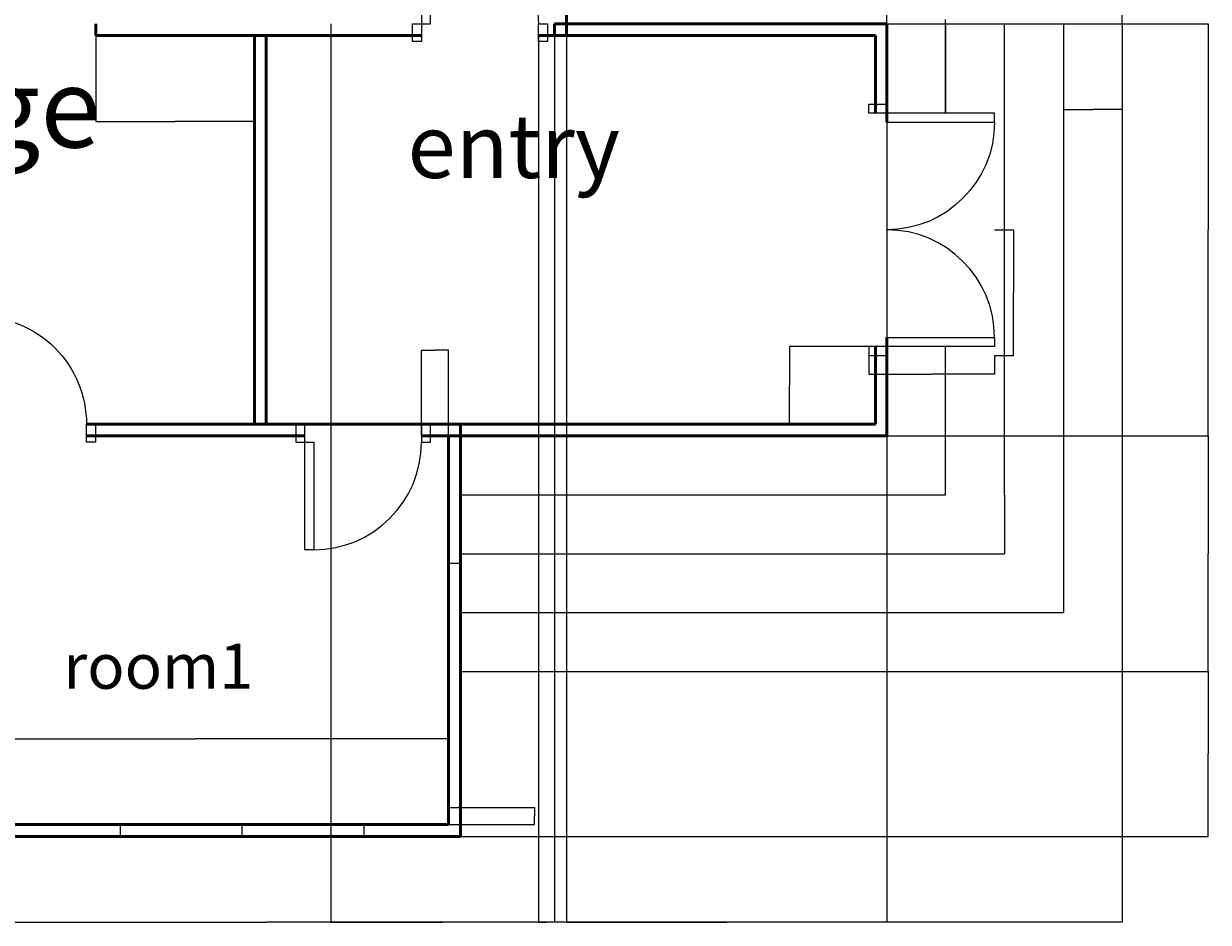
# Model space of a CAD drawing. Units: millimetres. Extents: x 756 to 17937, y 31 to 15590.
# Tile 3 of 6: x 7469 to 17520, y 31 to 7660. Entities that reach past the tile are written whole.
import ezdxf

# ---------------------------------------------------------------- set-up
doc = ezdxf.new("R2010")
doc.units = ezdxf.units.MM
for name, color, linetype, lineweight in [('A-ANNO-DIMS', 2, 'Continuous', 18), ('A-AREA-IDEN', 7, 'Continuous', 25), ('A-DOOR', 3, 'Continuous', 25), ('A-FLOR-STRS', 7, 'Continuous', 25), ('A-GLAZ', 4, 'Continuous', 18), ('A-WALL', 7, 'Continuous', 50)]:
    doc.layers.add(name, color=color, linetype=linetype, lineweight=lineweight)
doc.styles.get("Standard").update_dxf_attribs({"font": 'arial.ttf'})
doc.dimstyles.get("Standard").update_dxf_attribs({"dimtxt": 0.18, "dimasz": 0.18, "dimexe": 0.18, "dimexo": 0.0625, "dimgap": 0.09, "dimtad": 0, "dimtih": 1, "dimtoh": 1, "dimdec": 4, "dimzin": 0, "dimdsep": 46, "dimtxsty": 'Standard', "dimcen": 0.09, "dimadec": 0, "dimazin": 0, "dimtfac": 1, "dimtdec": 4, "dimtofl": 0, "dimtmove": 0, "dimatfit": 3, "dimfxl": 1, "dimtolj": 1, "dimtzin": 0, "dimarcsym": 0})

# ---------------------------------------------------------------- blocks, each defined once
blk = doc.blocks.new('DOOR-SINGLE-914')
for p, q in [((76.2004154520555, 1066.800209260013), (0.0004154520547672, 1066.800209260013)), ((0.0004154520547672, 1066.800209260013), (0.0004154520547672, 914.400209260013)), ((76.2004154520555, 914.400209260013), (76.2004154520555, 1066.800209260013)), ((1143.000415452054, 1066.800209260013), (1066.800415452054, 1066.800209260013)), ((1066.800415452054, 1066.800209260013), (1066.800415452054, 914.400209260013)), ((1143.000415452054, 914.400209260013), (1143.000415452054, 1066.800209260013)), ((0.0004154520547672, 914.400209260013), (76.2004154520555, 914.400209260013)), ((76.2004154520555, 914.400209260013), (152.4004154520562, 914.400209260013)), ((76.2004154520555, 0.0002092600134347), (76.2004154520555, 914.400209260013)), ((152.4004154520562, 914.400209260013), (152.4004154520562, 0.0002092600134347)), ((1066.800415452054, 914.400209260013), (1143.000415452054, 914.400209260013)), ((152.4004154520562, 0.0002092600134347), (76.2004154520555, 0.0002092600134347))]:
    blk.add_line(p, q)
blk.add_arc((152.4004154520562, 914.400209260013), 914.3999999999996, 270, 0)
blk = doc.blocks.new('DOOR-PAIR-LEAF-914')
for p, q in [((152.4003917740337, 76.20024496712995), (152.4003917740337, 152.4002449671306)), ((152.4003917740337, 152.4002449671306), (1066.800391774033, 152.4002449671306)), ((1066.800391774033, 152.4002449671306), (1066.800391774033, 76.20024496712995)), ((152.4003917740337, 76.20024496712995), (0.0003917740341421, 76.20024496712995)), ((0.0003917740341421, 76.20024496712995), (0.0003917740341421, 0.0002449671292197)), ((0.0003917740341421, 0.0002449671292197), (152.4003917740337, 0.0002449671292197)), ((1066.800391774033, 76.20024496712995), (152.4003917740337, 76.20024496712995)), ((152.4003917740337, 0.0002449671292197), (152.4003917740337, 76.20024496712995))]:
    blk.add_line(p, q)
blk.add_arc((152.4003917740337, 152.4002449671306), 914.3999999999996, 0, 90)
blk = doc.blocks.new('WIN-2073')
for p, q in [((8.2799133452e-06, 99.99960647437545), (8.2799133452e-06, -0.0003935256245313)), ((2072.903750917166, 99.99960647437545), (8.2799133452e-06, 99.99960647437545)), ((2072.903750917166, -0.0003935256245313), (2072.903750917166, 99.99960647437545)), ((8.2799133452e-06, -0.0003935256245313), (2072.903750917166, -0.0003935256245313))]:
    blk.add_line(p, q)
blk = doc.blocks.new('*D19')
at = {"layer": 'A-ANNO-DIMS', "color": 0, "lineweight": -2, "transparency": 16777216}
for p, q in [((15706.70389177404, 5910.170244967132), (15866.84139177405, 5910.170244967132)), ((15866.66139177405, 5909.990244967132), (15866.66139177405, 5376.952148104922)), ((15866.66139177405, 4843.550244967131), (15866.66139177405, 5376.588341829341)), ((15706.70389177404, 4843.370244967131), (15866.84139177405, 4843.370244967131))]:
    blk.add_line(p, q, dxfattribs=at)
at = {"layer": 'A-ANNO-DIMS', "color": 0, "transparency": 16777216}
for points in [[(15866.63139177405, 5909.990244967132), (15866.69139177405, 5909.990244967132), (15866.66139177405, 5910.170244967132)], [(15866.63139177405, 4843.550244967131), (15866.69139177405, 4843.550244967131), (15866.66139177405, 4843.370244967131)]]:
    blk.add_solid(points, dxfattribs=at)
at = {"layer": 'Defpoints', "color": 0, "transparency": 16777216}
for p in [(15706.64139177404, 5910.170244967132), (15866.66139177405, 5910.170244967132), (15706.64139177404, 4843.370244967131)]:
    blk.add_point(p, dxfattribs=at)
at = {"layer": 'A-ANNO-DIMS', "color": 0, "transparency": 16777216, "insert": (15866.66139177405, 5376.770244967126), "char_height": 0.18, "attachment_point": 5}
blk.add_mtext('\\A1;PAIRED LEAF 1067 TYP.', dxfattribs=at)
blk = doc.blocks.new('*D20')
at = {"layer": 'A-ANNO-DIMS', "color": 0, "lineweight": -2, "transparency": 16777216}
for p, q in [((14639.84139177403, 4843.30774496713), (14639.84139177403, 4683.170244967128)), ((15706.64139177403, 4843.30774496713), (15706.64139177403, 4683.170244967128)), ((14640.02139177403, 4683.350244967129), (15172.58192383406, 4683.350244967129)), ((15706.46139177403, 4683.350244967129), (15173.90085971401, 4683.350244967129))]:
    blk.add_line(p, q, dxfattribs=at)
at = {"layer": 'A-ANNO-DIMS', "color": 0, "transparency": 16777216}
for points in [[(14640.02139177403, 4683.380244967128), (14640.02139177403, 4683.320244967129), (14639.84139177403, 4683.350244967129)], [(15706.46139177403, 4683.380244967128), (15706.46139177403, 4683.320244967129), (15706.64139177403, 4683.350244967129)]]:
    blk.add_solid(points, dxfattribs=at)
at = {"layer": 'Defpoints', "color": 0, "transparency": 16777216}
for p in [(14639.84139177403, 4843.370244967129), (15706.64139177403, 4843.370244967129), (15706.64139177403, 4683.350244967129)]:
    blk.add_point(p, dxfattribs=at)
at = {"layer": 'A-ANNO-DIMS', "color": 0, "transparency": 16777216, "insert": (15173.24139177403, 4683.350244967129), "char_height": 0.18, "attachment_point": 5}
blk.add_mtext('\\A1;1067 TYP.', dxfattribs=at)
blk = doc.blocks.new('*D43')
at = {"layer": 'A-ANNO-DIMS', "color": 0, "lineweight": -2, "transparency": 16777216}
for p, q in [((16790.928101, 2160.118106), (16790.928101, 30.75060600000006)), ((2274.113703, 760.118106), (2274.113703, 30.75060600000006)), ((2274.293703, 30.930606), (9532.10067689768, 30.930606)), ((16790.748101, 30.930606), (9532.94112710232, 30.930606))]:
    blk.add_line(p, q, dxfattribs=at)
at = {"layer": 'A-ANNO-DIMS', "color": 0, "transparency": 16777216}
for points in [[(2274.293703, 30.960606), (2274.293703, 30.900606), (2274.113703, 30.930606)], [(16790.748101, 30.960606), (16790.748101, 30.900606), (16790.928101, 30.930606)]]:
    blk.add_solid(points, dxfattribs=at)
at = {"layer": 'Defpoints', "color": 0, "transparency": 16777216}
for p in [(16790.928101, 2160.180606), (2274.113703, 760.180606), (16790.928101, 30.930606)]:
    blk.add_point(p, dxfattribs=at)
at = {"layer": 'A-ANNO-DIMS', "color": 0, "transparency": 16777216, "insert": (9532.520901999998, 30.930606), "char_height": 0.18, "attachment_point": 5}
blk.add_mtext('\\A1;14517', dxfattribs=at)
blk = doc.blocks.new('*D46')
at = {"layer": 'A-ANNO-DIMS', "color": 0, "lineweight": -2, "transparency": 16777216}
for p, q in [((6774.113703000001, 860.243106), (6774.113703000001, 1589.610606)), ((6774.293703000001, 1589.430606), (8923.751615687586, 1589.430606)), ((11073.933703, 1589.430606), (8924.475790312415, 1589.430606)), ((11074.113703, 860.243106), (11074.113703, 1589.610606))]:
    blk.add_line(p, q, dxfattribs=at)
at = {"layer": 'A-ANNO-DIMS', "color": 0, "transparency": 16777216}
for points in [[(6774.293703000001, 1589.460606), (6774.293703000001, 1589.400606), (6774.113703000001, 1589.430606)], [(11073.933703, 1589.460606), (11073.933703, 1589.400606), (11074.113703, 1589.430606)]]:
    blk.add_solid(points, dxfattribs=at)
at = {"layer": 'Defpoints', "color": 0, "transparency": 16777216}
for p in [(11074.113703, 1589.430606), (6774.113703000001, 860.1806059999999), (11074.113703, 860.1806059999999)]:
    blk.add_point(p, dxfattribs=at)
at = {"layer": 'A-ANNO-DIMS', "color": 0, "transparency": 16777216, "insert": (8924.113703, 1589.430606), "char_height": 0.18, "attachment_point": 5}
blk.add_mtext('\\A1;4300', dxfattribs=at)
blk = doc.blocks.new('*D47')
at = {"layer": 'A-ANNO-DIMS', "color": 0, "lineweight": -2, "transparency": 16777216}
for p, q in [((16790.99060100001, 2160.180606000001), (17520.35810100001, 2160.180606000001)), ((17520.17810100001, 2160.000606000002), (17520.17810100001, 1460.362509137791)), ((17520.17810100001, 760.3606060000012), (17520.17810100001, 1459.998702862211)), ((11174.176203, 760.1806060000002), (17520.35810100001, 760.1806060000011))]:
    blk.add_line(p, q, dxfattribs=at)
at = {"layer": 'A-ANNO-DIMS', "color": 0, "transparency": 16777216}
for points in [[(17520.14810100001, 2160.000606000002), (17520.20810100001, 2160.000606000002), (17520.17810100001, 2160.180606000001)], [(17520.14810100001, 760.3606060000012), (17520.20810100001, 760.3606060000012), (17520.17810100001, 760.1806060000011)]]:
    blk.add_solid(points, dxfattribs=at)
at = {"layer": 'Defpoints', "color": 0, "transparency": 16777216}
for p in [(16790.92810100001, 2160.180606000001), (17520.17810100001, 2160.180606000001), (11174.113703, 760.1806060000002)]:
    blk.add_point(p, dxfattribs=at)
at = {"layer": 'A-ANNO-DIMS', "color": 0, "transparency": 16777216, "insert": (17520.17810100001, 1460.180605999996), "char_height": 0.18, "attachment_point": 5}
blk.add_mtext('\\A1;1400', dxfattribs=at)
blk = doc.blocks.new('*D48')
at = {"layer": 'A-ANNO-DIMS', "color": 0, "lineweight": -2, "transparency": 16777216}
for p, q in [((14792.303892, 4160.180606000001), (17520.35810100001, 4160.180606000001)), ((17520.17810100001, 4160.000606000001), (17520.17810100001, 3160.362509137792)), ((17520.17810100001, 2160.360606000001), (17520.17810100001, 3159.998702862212)), ((16790.99060100001, 2160.180606000001), (17520.35810100001, 2160.180606000001))]:
    blk.add_line(p, q, dxfattribs=at)
at = {"layer": 'A-ANNO-DIMS', "color": 0, "transparency": 16777216}
for points in [[(17520.14810100001, 4160.000606000001), (17520.20810100001, 4160.000606000001), (17520.17810100001, 4160.180606000001)], [(17520.14810100001, 2160.360606000001), (17520.20810100001, 2160.360606000001), (17520.17810100001, 2160.180606000001)]]:
    blk.add_solid(points, dxfattribs=at)
at = {"layer": 'Defpoints', "color": 0, "transparency": 16777216}
for p in [(14792.241392, 4160.180606000001), (17520.17810100001, 4160.180606000001), (16790.92810100001, 2160.180606000001)]:
    blk.add_point(p, dxfattribs=at)
at = {"layer": 'A-ANNO-DIMS', "color": 0, "transparency": 16777216, "insert": (17520.17810100001, 3160.180605999996), "char_height": 0.18, "attachment_point": 5}
blk.add_mtext('\\A1;2000', dxfattribs=at)
blk = doc.blocks.new('*D49')
at = {"layer": 'A-ANNO-DIMS', "color": 0, "lineweight": -2, "transparency": 16777216}
for p, q in [((14792.303892, 7660.159883000004), (17520.35810100001, 7660.159883000004)), ((17520.17810100001, 7659.979883000004), (17520.17810100001, 5910.352209029333)), ((17520.17810100001, 4160.360606000002), (17520.17810100001, 5909.98827997067)), ((14792.303892, 4160.180606000001), (17520.35810100001, 4160.180606000001))]:
    blk.add_line(p, q, dxfattribs=at)
at = {"layer": 'A-ANNO-DIMS', "color": 0, "transparency": 16777216}
for points in [[(17520.14810100001, 7659.979883000004), (17520.20810100001, 7659.979883000004), (17520.17810100001, 7660.159883000004)], [(17520.14810100001, 4160.360606000002), (17520.20810100001, 4160.360606000002), (17520.17810100001, 4160.180606000001)]]:
    blk.add_solid(points, dxfattribs=at)
at = {"layer": 'Defpoints', "color": 0, "transparency": 16777216}
for p in [(14792.241392, 7660.159883000004), (17520.17810100001, 7660.159883000004), (14792.241392, 4160.180606000001)]:
    blk.add_point(p, dxfattribs=at)
at = {"layer": 'A-ANNO-DIMS', "color": 0, "transparency": 16777216, "insert": (17520.17810100001, 5910.170244499997), "char_height": 0.18, "attachment_point": 5}
blk.add_mtext('\\A1;3500', dxfattribs=at)
blk = doc.blocks.new('*D57')
at = {"layer": 'A-ANNO-DIMS', "color": 0, "lineweight": -2, "transparency": 16777216}
for p, q in [((14792.241392, 7660.097383), (14792.241392, 30.75060599999961)), ((12074.113703, 7560.097383), (12074.113703, 30.75060599999961)), ((12074.293703, 30.930606), (13432.81705636766, 30.930606)), ((14792.061392, 30.930606), (13433.53803863233, 30.930606))]:
    blk.add_line(p, q, dxfattribs=at)
at = {"layer": 'A-ANNO-DIMS', "color": 0, "transparency": 16777216}
for points in [[(12074.293703, 30.960606), (12074.293703, 30.900606), (12074.113703, 30.930606)], [(14792.061392, 30.960606), (14792.061392, 30.900606), (14792.241392, 30.930606)]]:
    blk.add_solid(points, dxfattribs=at)
at = {"layer": 'Defpoints', "color": 0, "transparency": 16777216}
for p in [(14792.241392, 7660.159883), (12074.113703, 7560.159883), (14792.241392, 30.930606)]:
    blk.add_point(p, dxfattribs=at)
at = {"layer": 'A-ANNO-DIMS', "color": 0, "transparency": 16777216, "insert": (13433.1775475, 30.930606), "char_height": 0.18, "attachment_point": 5}
blk.add_mtext('\\A1;2718', dxfattribs=at)
blk = doc.blocks.new('*D58')
at = {"layer": 'A-ANNO-DIMS', "color": 0, "lineweight": -2, "transparency": 16777216}
for p, q in [((14792.241392, 7660.222383), (14792.241392, 8389.589883)), ((14792.421392, 8389.409883), (15791.1295896105, 8389.409883)), ((16790.748101, 8389.409883), (15792.03990338949, 8389.409883)), ((16790.928101, 7660.222383), (16790.928101, 8389.589883))]:
    blk.add_line(p, q, dxfattribs=at)
at = {"layer": 'A-ANNO-DIMS', "color": 0, "transparency": 16777216}
for points in [[(14792.421392, 8389.439883000001), (14792.421392, 8389.379883), (14792.241392, 8389.409883)], [(16790.748101, 8389.439883000001), (16790.748101, 8389.379883), (16790.928101, 8389.409883)]]:
    blk.add_solid(points, dxfattribs=at)
at = {"layer": 'Defpoints', "color": 0, "transparency": 16777216}
for p in [(16790.928101, 8389.409883), (14792.241392, 7660.159883), (16790.928101, 7660.159883)]:
    blk.add_point(p, dxfattribs=at)
at = {"layer": 'A-ANNO-DIMS', "color": 0, "transparency": 16777216, "insert": (15791.5847465, 8389.409883), "char_height": 0.18, "attachment_point": 5}
blk.add_mtext('\\A1;1998.7', dxfattribs=at)
blk = doc.blocks.new('*D59')
at = {"layer": 'A-ANNO-DIMS', "color": 0, "lineweight": -2, "transparency": 16777216}
for p, q in [((16290.928101, 7660.097383), (16290.928101, 6930.729882999999)), ((16790.928101, 7660.097383), (16790.928101, 6930.729883000001)), ((16291.108101, 6930.909882999999), (16540.63956075443, 6930.909883000001)), ((16790.748101, 6930.909883000001), (16541.21664124556, 6930.909883000001))]:
    blk.add_line(p, q, dxfattribs=at)
at = {"layer": 'A-ANNO-DIMS', "color": 0, "transparency": 16777216}
for points in [[(16291.108101, 6930.939882999999), (16291.108101, 6930.879883), (16290.928101, 6930.909882999999)], [(16790.748101, 6930.939883), (16790.748101, 6930.879883000002), (16790.928101, 6930.909883000001)]]:
    blk.add_solid(points, dxfattribs=at)
at = {"layer": 'Defpoints', "color": 0, "transparency": 16777216}
for p in [(16290.928101, 7660.159883), (16790.928101, 7660.159883), (16290.928101, 6930.909882999999)]:
    blk.add_point(p, dxfattribs=at)
at = {"layer": 'A-ANNO-DIMS', "color": 0, "transparency": 16777216, "insert": (16540.928101, 6930.909883000001), "char_height": 0.18, "attachment_point": 5}
blk.add_mtext('\\A1;500', dxfattribs=at)
blk = doc.blocks.new('*D60')
at = {"layer": 'A-ANNO-DIMS', "color": 0, "lineweight": -2, "transparency": 16777216}
for p, q in [((8080.230142000001, 7560.118106), (8080.230142000001, 6830.750605999999)), ((9426.842559999997, 7560.118106), (9426.842559999997, 6830.750605999999)), ((8080.410142000001, 6830.930605999999), (8753.081255502046, 6830.930605999999)), ((9426.662559999999, 6830.930605999999), (8753.991446497952, 6830.930605999999))]:
    blk.add_line(p, q, dxfattribs=at)
at = {"layer": 'A-ANNO-DIMS', "color": 0, "transparency": 16777216}
for points in [[(8080.410142000001, 6830.960605999999), (8080.410142000001, 6830.900606), (8080.230142000001, 6830.930605999999)], [(9426.662559999999, 6830.960605999999), (9426.662559999999, 6830.900606), (9426.842559999997, 6830.930605999999)]]:
    blk.add_solid(points, dxfattribs=at)
at = {"layer": 'Defpoints', "color": 0, "transparency": 16777216}
for p in [(8080.230142000001, 7560.180606), (9426.842559999997, 7560.180606), (8080.230142000001, 6830.930605999999)]:
    blk.add_point(p, dxfattribs=at)
at = {"layer": 'A-ANNO-DIMS', "color": 0, "transparency": 16777216, "insert": (8753.536350999999, 6830.930605999999), "char_height": 0.18, "attachment_point": 5}
blk.add_mtext('\\A1;1346.6', dxfattribs=at)
blk = doc.blocks.new('*D62')
at = {"layer": 'A-ANNO-DIMS', "color": 0, "lineweight": -2, "transparency": 16777216}
for p, q in [((10075.381538, 7660.118106), (10075.381538, 30.75060599999961)), ((11974.113703, 7660.118106), (11974.113703, 30.75060599999961)), ((10075.561538, 30.930606), (11024.2924636105, 30.930606)), ((11973.933703, 30.930606), (11025.20277738949, 30.930606))]:
    blk.add_line(p, q, dxfattribs=at)
at = {"layer": 'A-ANNO-DIMS', "color": 0, "transparency": 16777216}
for points in [[(10075.561538, 30.960606), (10075.561538, 30.900606), (10075.381538, 30.930606)], [(11973.933703, 30.960606), (11973.933703, 30.900606), (11974.113703, 30.930606)]]:
    blk.add_solid(points, dxfattribs=at)
at = {"layer": 'Defpoints', "color": 0, "transparency": 16777216}
for p in [(10075.381538, 7660.180606), (11974.113703, 7660.180606), (11974.113703, 30.930606)]:
    blk.add_point(p, dxfattribs=at)
at = {"layer": 'A-ANNO-DIMS', "color": 0, "transparency": 16777216, "insert": (11024.7476205, 30.930606), "char_height": 0.18, "attachment_point": 5}
blk.add_mtext('\\A1;1898.7', dxfattribs=at)
blk = doc.blocks.new('*D65')
at = {"layer": 'A-ANNO-DIMS', "color": 0, "lineweight": -2, "transparency": 16777216}
for p, q in [((11074.176203, 1004.779303), (11803.54370300001, 1004.779303)), ((11803.36370300001, 1004.599303), (11803.36370300001, 932.6618576377907)), ((11803.36370300001, 860.3606060000005), (11803.36370300001, 932.2980513622107)), ((11074.176203, 860.1806060000004), (11803.54370300001, 860.1806060000006))]:
    blk.add_line(p, q, dxfattribs=at)
at = {"layer": 'A-ANNO-DIMS', "color": 0, "transparency": 16777216}
for points in [[(11803.333703, 1004.599303), (11803.39370300001, 1004.599303), (11803.36370300001, 1004.779303)], [(11803.333703, 860.3606060000005), (11803.39370300001, 860.3606060000005), (11803.36370300001, 860.1806060000006)]]:
    blk.add_solid(points, dxfattribs=at)
at = {"layer": 'Defpoints', "color": 0, "transparency": 16777216}
for p in [(11074.113703, 1004.779303), (11074.113703, 860.1806060000004), (11803.36370300001, 860.1806060000006)]:
    blk.add_point(p, dxfattribs=at)
at = {"layer": 'A-ANNO-DIMS', "color": 0, "transparency": 16777216, "insert": (11803.363703, 932.479954499997), "char_height": 0.18, "attachment_point": 5}
blk.add_mtext('\\A1;144.6', dxfattribs=at)
blk = doc.blocks.new('*D68')
at = {"layer": 'A-ANNO-DIMS', "color": 0, "lineweight": -2, "transparency": 16777216}
for p, q in [((14696.49700700001, 4919.570245000002), (13967.12950700001, 4919.570245)), ((13967.30950700001, 4919.390245), (13967.30950700001, 4590.05732863779)), ((13967.30950700001, 4260.360606000001), (13967.30950700001, 4589.693522362209)), ((14696.49700700001, 4260.180606000001), (13967.12950700001, 4260.180606000001))]:
    blk.add_line(p, q, dxfattribs=at)
at = {"layer": 'A-ANNO-DIMS', "color": 0, "transparency": 16777216}
for points in [[(13967.27950700001, 4919.390245), (13967.33950700001, 4919.390245), (13967.30950700001, 4919.570245)], [(13967.27950700001, 4260.360606000001), (13967.33950700001, 4260.360606000001), (13967.30950700001, 4260.180606000001)]]:
    blk.add_solid(points, dxfattribs=at)
at = {"layer": 'Defpoints', "color": 0, "transparency": 16777216}
for p in [(13967.30950700001, 4919.570245), (14696.55950700001, 4919.570245000002), (14696.55950700001, 4260.180606000001)]:
    blk.add_point(p, dxfattribs=at)
at = {"layer": 'A-ANNO-DIMS', "color": 0, "transparency": 16777216, "insert": (13967.30950700001, 4589.875425499996), "char_height": 0.18, "attachment_point": 5}
blk.add_mtext('\\A1;659.4', dxfattribs=at)
blk = doc.blocks.new('*D74')
at = {"layer": 'A-ANNO-DIMS', "color": 0, "lineweight": -2, "transparency": 16777216}
for p, q in [((11836.191606, 7560.118106), (11836.191606, 30.75060599999961)), ((11974.113703, 7560.097383), (11974.113703, 30.75060599999961)), ((11836.371606, 30.930606), (11904.69841848363, 30.930606)), ((11973.933703, 30.930606), (11905.60689051637, 30.930606))]:
    blk.add_line(p, q, dxfattribs=at)
at = {"layer": 'A-ANNO-DIMS', "color": 0, "transparency": 16777216}
for points in [[(11836.371606, 30.960606), (11836.371606, 30.900606), (11836.191606, 30.930606)], [(11973.933703, 30.960606), (11973.933703, 30.900606), (11974.113703, 30.930606)]]:
    blk.add_solid(points, dxfattribs=at)
at = {"layer": 'Defpoints', "color": 0, "transparency": 16777216}
for p in [(11836.191606, 7560.180606), (11974.113703, 7560.159883), (11836.191606, 30.930606)]:
    blk.add_point(p, dxfattribs=at)
at = {"layer": 'A-ANNO-DIMS', "color": 0, "transparency": 16777216, "insert": (11905.1526545, 30.930606), "char_height": 0.18, "attachment_point": 5}
blk.add_mtext('\\A1;137.92', dxfattribs=at)
blk = doc.blocks.new('*D77')
at = {"layer": 'A-ANNO-DIMS', "color": 0, "lineweight": -2, "transparency": 16777216}
for p, q in [((10844.590989, 4160.243106), (10844.590989, 4889.610606)), ((10844.770989, 4889.430606), (10958.95643194816, 4889.430606)), ((11073.933703, 4889.430606), (10959.74826005184, 4889.430606)), ((11074.113703, 4160.243106), (11074.113703, 4889.610606))]:
    blk.add_line(p, q, dxfattribs=at)
at = {"layer": 'A-ANNO-DIMS', "color": 0, "transparency": 16777216}
for points in [[(10844.770989, 4889.460606), (10844.770989, 4889.400606), (10844.590989, 4889.430606)], [(11073.933703, 4889.460606), (11073.933703, 4889.400606), (11074.113703, 4889.430606)]]:
    blk.add_solid(points, dxfattribs=at)
at = {"layer": 'Defpoints', "color": 0, "transparency": 16777216}
for p in [(11074.113703, 4889.430606), (10844.590989, 4160.180605999999), (11074.113703, 4160.180605999999)]:
    blk.add_point(p, dxfattribs=at)
at = {"layer": 'A-ANNO-DIMS', "color": 0, "transparency": 16777216, "insert": (10959.352346, 4889.430606), "char_height": 0.18, "attachment_point": 5}
blk.add_mtext('\\A1;229.5', dxfattribs=at)

msp = doc.modelspace()

# ---------------------------------------------------------------- linework, layer by layer
at = {"layer": 'A-FLOR-STRS'}
for p, q in [((14792.24139177403, 7660.159883459883), (16790.92810071155, 7660.159883459884)), ((15290.92810071155, 6900.770244967131), (15290.92810071155, 7696.561903523863)), ((15290.92810071155, 7660.159883459883), (15290.92810071155, 6900.770244967131)), ((15290.92810071154, 6900.770244967131), (15290.92810071154, 7660.159883459883)), ((15790.92810071155, 3660.180606474378), (15790.92810071155, 7660.159883459884)), ((16290.92810071155, 7660.159883459883), (16290.92810071155, 2660.180606474377)), ((16790.92810071155, 7660.159883459884), (16790.92810071154, 2160.180606474376)), ((15290.92810071155, 3660.180606474379), (15290.92810071155, 4919.57024496713)), ((11174.11370251699, 4160.180606474376), (11174.11370251699, 3960.180606474377)), ((11174.11370251699, 3960.180606474377), (11174.11370251699, 3660.180606474377)), ((11174.11370251699, 3660.180606474377), (14790.92810071155, 3660.180606474377)), ((11174.11370251699, 3660.180606474377), (15290.92810071155, 3660.180606474379)), ((14790.92810071155, 3660.180606474377), (15290.92810071155, 3660.180606474377)), ((15790.92810071155, 3660.180606474378), (15790.92810071155, 3160.180606474376)), ((11174.11370251699, 3160.180606474377), (15790.92810071155, 3160.180606474377)), ((11174.11370251699, 2660.180606474377), (16290.92810071155, 2660.180606474377)), ((11174.11370251699, 2160.180606474376), (16790.92810071154, 2160.180606474376))]:
    msp.add_line(p, q, dxfattribs=at)
at = {"layer": 'A-WALL'}
for p, q in [((12074.11370251699, 14760.18060647437), (12074.11370251699, 7560.159883459885)), ((8080.230141901877, 7660.180606474376), (8080.230141901877, 7560.180606474377)), ((11974.11370251699, 7660.180606474376), (11974.11370251699, 7560.180606474375)), ((11974.11370251699, 7560.159883459883), (11974.11370251699, 7660.159883459883)), ((11974.11370251699, 7660.159883459883), (14692.24139177403, 7660.159883459883)), ((14692.24139177403, 7660.159883459883), (14792.24139177403, 7660.159883459883)), ((14792.24139177403, 7660.159883459883), (14792.24139177403, 6824.57024496713)), ((10845.59160552457, 7560.180606474375), (8080.230141901878, 7560.180606474377)), ((9526.84255957045, 7560.180606474377), (9426.84255957045, 7560.180606474377)), ((9426.84255957045, 7560.180606474377), (9426.84255957045, 4260.180606474377)), ((9526.842559570447, 4260.180606474377), (9526.84255957045, 7560.180606474377)), ((11974.11370251699, 7560.180606474375), (11836.19160552456, 7560.180606474375)), ((12074.11370251699, 7560.159883459885), (11974.11370251699, 7560.159883459883)), ((12074.11370251699, 7560.159883459885), (14696.55950712074, 7560.159883459885)), ((14696.55950712074, 7560.159883459885), (14696.55950712075, 7359.089164103498)), ((14696.55950712075, 6900.77024496713), (14696.55950712075, 7475.987621863315)), ((14792.24139177403, 4995.770244967132), (14792.24139177403, 4160.180606474376)), ((14696.55950712075, 4260.180606474377), (14696.55950712075, 4919.57024496713)), ((8002.131150071232, 4260.180606474377), (9853.990988645633, 4260.180606474377)), ((9426.84255957045, 4260.180606474377), (14696.55950712075, 4260.180606474377)), ((10844.59098864563, 4260.180606474377), (11174.11370251699, 4260.180606474377)), ((11174.11370251699, 4260.180606474377), (11174.11370251699, 4160.180606474376)), ((9853.990988645633, 4160.180606474376), (8002.131150071226, 4160.180606474376)), ((8002.131150071226, 4160.180606474376), (9853.990988645633, 4160.180606474376)), ((11074.11370251699, 4160.180606474376), (10844.59098864563, 4160.180606474376)), ((10844.59098864563, 4160.180606474376), (11174.11370251699, 4160.180606474376)), ((11074.11370251699, 860.1806064743769), (11074.11370251699, 4160.180606474376)), ((11174.11370251699, 4160.180606474376), (11174.11370251699, 860.1806064743769)), ((11174.11370251699, 4160.180606474376), (14792.24139177403, 4160.180606474376)), ((6674.11370251699, 860.1806064743769), (10974.11370251699, 860.1806064743769)), ((10974.11370251699, 860.1806064743769), (11074.11370251699, 860.1806064743769)), ((11174.11370251699, 860.1806064743769), (11174.11370251699, 760.1806064743769)), ((11174.11370251699, 760.1806064743769), (6874.11370251699, 760.1806064743769))]:
    msp.add_line(p, q, dxfattribs=at)

# ---------------------------------------------------------------- block references
at = {"layer": 'A-DOOR', "extrusion": (0, 0, -1), "zscale": -1, "rotation": 180}
for name, p in [('DOOR-SINGLE-914', (-10769.39119007251, 8574.58081573439)), ('DOOR-PAIR-LEAF-914', (-14639.841, 6976.970489934261)), ('DOOR-SINGLE-914', (-6935.330734619177, 5174.580815734389))]:
    msp.add_blockref(name, p, dxfattribs=at)
at = {"layer": 'A-DOOR'}
for name, p in [('DOOR-PAIR-LEAF-914', (14639.841, 4843.37)), ('DOOR-SINGLE-914', (9777.79057319358, 3193.380397214363))]:
    msp.add_blockref(name, p, dxfattribs=at)
at = {"layer": 'A-GLAZ', "rotation": 90.00000000000003}
msp.add_blockref('WIN-2073', (11174.11330899136, 1004.779294616087), dxfattribs=at)
at = {"layer": 'A-GLAZ'}
for p in [(7249.967394579387, 760.181000000006), (8286.419265898016, 760.181000000006)]:
    msp.add_blockref('WIN-2073', p, dxfattribs=at)

# ---------------------------------------------------------------- texts
at = {"layer": 'A-AREA-IDEN', "attachment_point": 1}
for s, width, gutter_width, insert, char_height in [('lounge', 8015.314607100638, 3380.596656314288, (5146.970008784338, 7285.034507218895), 676.1193312628575), ('entry', 8152.240441860875, 33.7103631331366, (10725.85331514926, 6889.611356744802), 539.3658101301857), ('room1', 5870.212435527328, 1919.122497311093, (7805.324190083296, 2397.398024502683), 383.8244994622185)]:
    msp.add_mtext_dynamic_manual_height_columns(s, width=width, gutter_width=gutter_width, heights=[0], dxfattribs=dict(at, insert=insert, char_height=char_height))

# ---------------------------------------------------------------- dimensions: what is measured, and where the dimension line sits
at = {"layer": 'A-ANNO-DIMS'}
for base, p1, p2, angle, override, picture, middle in [((16790.928101, 8389.409883), (14792.241392, 7660.159883), (16790.928101, 7660.159883), 5.21e-14, {"dimdec": 1, "dimlfac": 1, "dimrnd": 0, "dimzin": 0, "dimdsep": 46, "dimlunit": 2}, '*D58', (15791.5847465, 8389.409883)), ((17520.17810100001, 7660.159883000004), (14792.241392, 4160.180605999999), (14792.241392, 7660.159883), 90, {"dimdec": 0, "dimlfac": 1, "dimrnd": 0, "dimzin": 0, "dimdsep": 46, "dimlunit": 2}, '*D49', (17520.17810100001, 5910.170244499997)), ((16290.928101, 6930.909882999999), (16790.928101, 7660.159883), (16290.928101, 7660.159883), 180.0000000000002, {"dimdec": 0, "dimlfac": 1, "dimrnd": 0, "dimzin": 0, "dimdsep": 46, "dimlunit": 2}, '*D59', (16540.928101, 6930.909883000001)), ((8080.230142000001, 6830.930605999999), (9426.842559999997, 7560.180606), (8080.230142000001, 7560.180606), 180, {"dimdec": 1, "dimlfac": 1, "dimrnd": 0, "dimzin": 0, "dimdsep": 46, "dimlunit": 2}, '*D60', (8753.536350999999, 6830.930605999999)), ((13967.30950700001, 4919.570245), (14696.559507, 4260.180606), (14696.559507, 4919.570245), 90, {"dimdec": 1, "dimlfac": 1, "dimrnd": 0, "dimzin": 0, "dimdsep": 46, "dimlunit": 2}, '*D68', (13967.30950700001, 4589.875425499996)), ((17520.17810100001, 4160.180606000001), (16790.928101, 2160.180606), (14792.241392, 4160.180605999999), 90, {"dimdec": 0, "dimlfac": 1, "dimrnd": 0, "dimzin": 0, "dimdsep": 46, "dimlunit": 2}, '*D48', (17520.17810100001, 3160.180605999996)), ((17520.17810100001, 2160.180606000001), (11174.113703, 760.180606), (16790.928101, 2160.180606), 90, {"dimdec": 0, "dimlfac": 1, "dimrnd": 0, "dimzin": 0, "dimdsep": 46, "dimlunit": 2}, '*D47', (17520.17810100001, 1460.180605999996)), ((11803.36370300001, 860.1806060000006), (11074.113703, 1004.779303), (11074.113703, 860.1806059999999), 270.0000000000021, {"dimdec": 1, "dimlfac": 1, "dimrnd": 0, "dimzin": 0, "dimdsep": 46, "dimlunit": 2}, '*D65', (11803.363703, 932.479954499997))]:
    dim = msp.add_linear_dim(base=base, p1=p1, p2=p2, angle=angle, dimstyle='Standard', override=override, dxfattribs=at)
    dim.commit()
    dim.dimension.update_dxf_attribs({"geometry": picture, "text_midpoint": middle})
for base, p1, p2, override, picture, middle in [((11974.113703, 30.930606), (10075.381538, 7660.180606), (11974.113703, 7660.180606), {"dimdec": 1, "dimlfac": 1, "dimrnd": 0, "dimzin": 0, "dimdsep": 46, "dimlunit": 2}, '*D62', (11024.7476205, 30.930606)), ((14792.241392, 30.930606), (12074.113703, 7560.159883), (14792.241392, 7660.159883), {"dimdec": 0, "dimlfac": 1, "dimrnd": 0, "dimzin": 0, "dimdsep": 46, "dimlunit": 2}, '*D57', (13433.1775475, 30.930606)), ((11836.191606, 30.930606), (11974.113703, 7560.159883), (11836.191606, 7560.180606), {"dimdec": 2, "dimlfac": 1, "dimrnd": 0, "dimzin": 0, "dimdsep": 46, "dimlunit": 2}, '*D74', (11905.1526545, 30.930606)), ((11074.113703, 4889.430606), (10844.590989, 4160.180605999999), (11074.113703, 4160.180605999999), {"dimdec": 1, "dimlfac": 1, "dimrnd": 0, "dimzin": 0, "dimdsep": 46, "dimlunit": 2}, '*D77', (10959.352346, 4889.430606)), ((16790.928101, 30.930606), (2274.113703, 760.180606), (16790.928101, 2160.180606), {"dimdec": 0, "dimlfac": 1, "dimrnd": 0, "dimzin": 0, "dimdsep": 46, "dimlunit": 2}, '*D43', (9532.520901999998, 30.930606)), ((11074.113703, 1589.430606), (6774.113703000001, 860.1806059999999), (11074.113703, 860.1806059999999), {"dimdec": 0, "dimlfac": 1, "dimrnd": 0, "dimzin": 0, "dimdsep": 46, "dimlunit": 2}, '*D46', (8924.113703, 1589.430606))]:
    dim = msp.add_linear_dim(base=base, p1=p1, p2=p2, dimstyle='Standard', override=override, dxfattribs=at)
    dim.commit()
    dim.dimension.update_dxf_attribs({"geometry": picture, "text_midpoint": middle})
dim = msp.add_linear_dim(base=(15866.66139177405, 5910.170244967132), p1=(15706.64139177403, 4843.370244967129), p2=(15706.64139177403, 5910.17024496713), angle=90, text='PAIRED LEAF <> TYP.', dimstyle='Standard', override={"dimdec": 0, "dimlfac": 1, "dimrnd": 0, "dimzin": 0, "dimdsep": 46, "dimlunit": 2}, dxfattribs=at)
dim.commit()
dim.dimension.update_dxf_attribs({"geometry": '*D19', "text_midpoint": (15866.66139177405, 5376.770244967126)})
dim = msp.add_linear_dim(base=(15706.64139177403, 4683.350244967129), p1=(14639.84139177403, 4843.370244967129), p2=(15706.64139177403, 4843.370244967129), text='<> TYP.', dimstyle='Standard', override={"dimdec": 0, "dimlfac": 1, "dimrnd": 0, "dimzin": 0, "dimdsep": 46, "dimlunit": 2}, dxfattribs=at)
dim.commit()
dim.dimension.update_dxf_attribs({"geometry": '*D20', "text_midpoint": (15173.24139177403, 4683.350244967129)})

doc.saveas('drawing.dxf')
